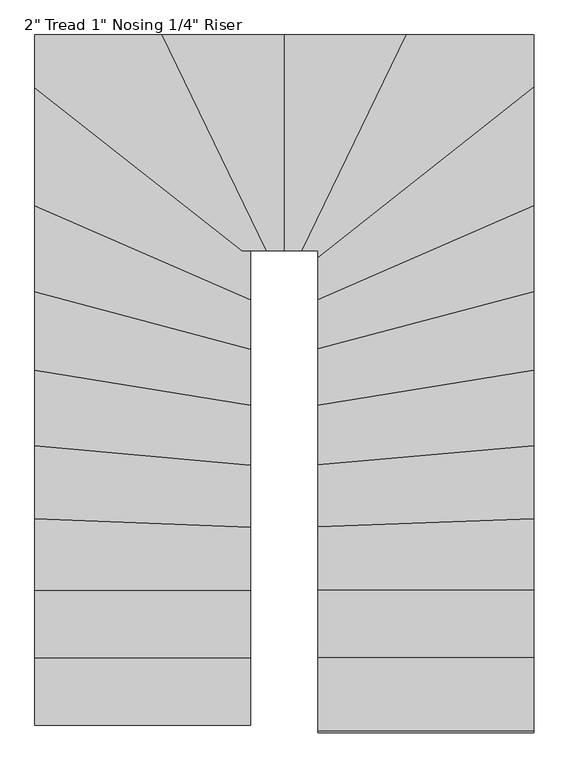
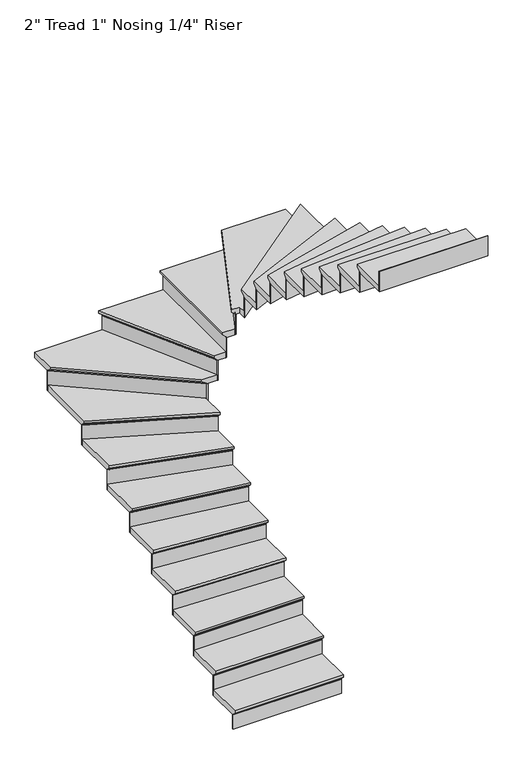
"""IFC4 building model written with IfcOpenShell, lengths in millimetres: stair flight geometry."""

from ifc_helpers import new_model, si_unit, origin, place, context, project, spatial, faceted_brep, source, transform, mapped, element, save


def stair_flight_652fc51c(model_context):
    return source(origin(), model_context, "Body", "Brep", [
        faceted_brep([(-5047.1987704, -4554.2130548, 22100.7214286), (-5047.1987704, -4554.2130548, 22119.7714286), (-5940.8822214, -4554.2130548, 22119.7714286), (-5940.8822214, -4554.2130548, 22100.7214286), (-5047.1987704, -4528.8130548, 22075.3214286), (-5940.8822214, -4528.8130548, 22075.3214286), (-5047.1987704, -4249.4130548, 22119.7714286), (-5940.8822214, -4249.4130548, 22119.7714286), (-5940.8822214, -4528.8130548, 22068.9714286), (-5940.8822214, -4249.4130548, 22068.9714286), (-5047.1987704, -4249.4130548, 22068.9714286), (-5047.1987704, -4528.8130548, 22068.9714286)], [[[0, 1, 2, 3]], [[4, 0, 3, 5]], [[2, 1, 6, 7]], [[8, 9, 10, 11]], [[2, 7, 9, 8, 5, 3]], [[8, 11, 4, 5]], [[6, 1, 0, 4, 11, 10]], [[7, 6, 10, 9]]]),
        faceted_brep([(-5047.1987704, -4528.8130548, 22068.9714286), (-5047.1987704, -4528.8130548, 21945.6), (-5047.1987704, -4522.4630548, 21945.6), (-5047.1987704, -4522.4630548, 22068.9714286), (-5940.8822214, -4528.8130548, 22068.9714286), (-5940.8822214, -4522.4630548, 22068.9714286), (-5940.8822214, -4522.4630548, 21945.6), (-5940.8822214, -4528.8130548, 21945.6)], [[[0, 1, 2, 3]], [[4, 5, 6, 7]], [[1, 0, 4, 7]], [[2, 1, 7, 6]], [[3, 2, 6, 5]], [[0, 3, 5, 4]]]),
        faceted_brep([(-5047.1987704, -4249.4130548, 22243.1428571), (-5047.1987704, -4249.4130548, 22068.9714286), (-5047.1987704, -4243.0630548, 22068.9714286), (-5047.1987704, -4243.0630548, 22243.1428571), (-5940.8822214, -4249.4130548, 22243.1428571), (-5940.8822214, -4243.0630548, 22243.1428571), (-5940.8822214, -4243.0630548, 22068.9714286), (-5940.8822214, -4249.4130548, 22068.9714286)], [[[0, 1, 2, 3]], [[4, 5, 6, 7]], [[1, 0, 4, 7]], [[2, 1, 7, 6]], [[3, 2, 6, 5]], [[0, 3, 5, 4]]]),
        faceted_brep([(-5940.8822214, -4274.8130548, 22293.9428571), (-5047.1987704, -4274.8130548, 22293.9428571), (-5047.1987704, -3970.0130548, 22293.9428571), (-5940.8822214, -3970.0130548, 22293.9428571), (-5940.8822214, -4249.4130548, 22243.1428571), (-5940.8822214, -3970.0130548, 22243.1428571), (-5047.1987704, -3970.0130548, 22243.1428571), (-5047.1987704, -4249.4130548, 22243.1428571), (-5940.8822214, -4249.4130548, 22249.4928571), (-5940.8822214, -4274.8130548, 22274.8928571), (-5047.1987704, -4249.4130548, 22249.4928571), (-5047.1987704, -4274.8130548, 22274.8928571)], [[[0, 1, 2, 3]], [[4, 5, 6, 7]], [[0, 3, 5, 4, 8, 9]], [[4, 7, 10, 8]], [[2, 1, 11, 10, 7, 6]], [[3, 2, 6, 5]], [[11, 1, 0, 9]], [[10, 11, 9, 8]]]),
        faceted_brep([(-5047.1987704, -3970.0130548, 22417.3142857), (-5047.1987704, -3970.0130548, 22243.1428571), (-5047.1987704, -3963.6630548, 22243.1428571), (-5047.1987704, -3963.6630548, 22417.3142857), (-5940.8822214, -3970.0130548, 22417.3142857), (-5940.8822214, -3963.6630548, 22417.3142857), (-5940.8822214, -3963.6630548, 22243.1428571), (-5940.8822214, -3970.0130548, 22243.1428571)], [[[0, 1, 2, 3]], [[4, 5, 6, 7]], [[1, 0, 4, 7]], [[2, 1, 7, 6]], [[3, 2, 6, 5]], [[0, 3, 5, 4]]]),
        faceted_brep([(-5940.8822214, -3995.4130548, 22468.1142857), (-5047.1987704, -3995.4130548, 22468.1142857), (-5047.1987704, -3707.9036879, 22468.1142857), (-5940.8822214, -3673.2843203, 22468.1142857), (-5940.8822214, -3970.0130548, 22417.3142857), (-5940.8822214, -3673.2843203, 22417.3142857), (-5047.1987704, -3707.9036879, 22417.3142857), (-5047.1987704, -3970.0130548, 22417.3142857), (-5940.8822214, -3970.0130548, 22423.6642857), (-5940.8822214, -3995.4130548, 22449.0642857), (-5047.1987704, -3970.0130548, 22423.6642857), (-5047.1987704, -3995.4130548, 22449.0642857)], [[[0, 1, 2, 3]], [[4, 5, 6, 7]], [[0, 3, 5, 4, 8, 9]], [[4, 7, 10, 8]], [[2, 1, 11, 10, 7, 6]], [[3, 2, 6, 5]], [[11, 1, 0, 9]], [[10, 11, 9, 8]]]),
        faceted_brep([(-5047.1987704, -3707.9036879, 22591.4857143), (-5047.1987704, -3707.9036879, 22417.3142857), (-5047.1987704, -3701.5489252, 22417.3142857), (-5047.1987704, -3701.5489252, 22591.4857143), (-5940.8822214, -3673.2843203, 22591.4857143), (-5940.8822214, -3666.9295576, 22591.4857143), (-5940.8822214, -3666.9295576, 22417.3142857), (-5940.8822214, -3673.2843203, 22417.3142857)], [[[0, 1, 2, 3]], [[4, 5, 6, 7]], [[1, 0, 4, 7]], [[2, 1, 7, 6]], [[3, 2, 6, 5]], [[0, 3, 5, 4]]]),
        faceted_brep([(-5940.8822214, -3698.703371, 22642.2857143), (-5047.1987704, -3733.3227386, 22642.2857143), (-5047.1987704, -3451.3234819, 22642.2857143), (-5940.8822214, -3370.89733, 22642.2857143), (-5940.8822214, -3673.2843203, 22591.4857143), (-5940.8822214, -3370.89733, 22591.4857143), (-5047.1987704, -3451.3234819, 22591.4857143), (-5047.1987704, -3707.9036879, 22591.4857143), (-5940.8822214, -3673.2843203, 22597.8357143), (-5940.8822214, -3698.703371, 22623.2357143), (-5047.1987704, -3707.9036879, 22597.8357143), (-5047.1987704, -3733.3227386, 22623.2357143)], [[[0, 1, 2, 3]], [[4, 5, 6, 7]], [[0, 3, 5, 4, 8, 9]], [[4, 7, 10, 8]], [[2, 1, 11, 10, 7, 6]], [[3, 2, 6, 5]], [[11, 1, 0, 9]], [[10, 11, 9, 8]]]),
        faceted_brep([(-5047.1987704, -3451.3234819, 22765.6571429), (-5047.1987704, -3451.3234819, 22591.4857143), (-5047.1987704, -3444.9478197, 22591.4857143), (-5047.1987704, -3444.9478197, 22765.6571429), (-5940.8822214, -3370.89733, 22765.6571429), (-5940.8822214, -3364.5216678, 22765.6571429), (-5940.8822214, -3364.5216678, 22591.4857143), (-5940.8822214, -3370.89733, 22591.4857143)], [[[0, 1, 2, 3]], [[4, 5, 6, 7]], [[1, 0, 4, 7]], [[2, 1, 7, 6]], [[3, 2, 6, 5]], [[0, 3, 5, 4]]]),
        faceted_brep([(-5940.8822214, -3396.3999789, 22816.4571429), (-5047.1987704, -3476.8261308, 22816.4571429), (-5047.1987704, -3203.4301079, 22816.4571429), (-5940.8822214, -3059.5417727, 22816.4571429), (-5940.8822214, -3370.89733, 22765.6571429), (-5940.8822214, -3059.5417727, 22765.6571429), (-5047.1987704, -3203.4301079, 22765.6571429), (-5047.1987704, -3451.3234819, 22765.6571429), (-5940.8822214, -3370.89733, 22772.0071429), (-5940.8822214, -3396.3999789, 22797.4071429), (-5047.1987704, -3451.3234819, 22772.0071429), (-5047.1987704, -3476.8261308, 22797.4071429)], [[[0, 1, 2, 3]], [[4, 5, 6, 7]], [[0, 3, 5, 4, 8, 9]], [[4, 7, 10, 8]], [[2, 1, 11, 10, 7, 6]], [[3, 2, 6, 5]], [[11, 1, 0, 9]], [[10, 11, 9, 8]]]),
        faceted_brep([(-5047.1987704, -3203.4301079, 22939.8285714), (-5047.1987704, -3203.4301079, 22765.6571429), (-5047.1987704, -3196.9983292, 22765.6571429), (-5047.1987704, -3196.9983292, 22939.8285714), (-5940.8822214, -3059.5417727, 22939.8285714), (-5940.8822214, -3053.109994, 22939.8285714), (-5940.8822214, -3053.109994, 22765.6571429), (-5940.8822214, -3059.5417727, 22765.6571429)], [[[0, 1, 2, 3]], [[4, 5, 6, 7]], [[1, 0, 4, 7]], [[2, 1, 7, 6]], [[3, 2, 6, 5]], [[0, 3, 5, 4]]]),
        faceted_brep([(-5940.8822214, -3085.2688872, 22990.6285714), (-5047.1987704, -3229.1572224, 22990.6285714), (-5047.1987704, -2970.3553609, 22990.6285714), (-5940.8822214, -2732.7052783, 22990.6285714), (-5940.8822214, -3059.5417727, 22939.8285714), (-5940.8822214, -2732.7052783, 22939.8285714), (-5047.1987704, -2970.3553609, 22939.8285714), (-5047.1987704, -3203.4301079, 22939.8285714), (-5940.8822214, -3059.5417727, 22946.1785714), (-5940.8822214, -3085.2688872, 22971.5785714), (-5047.1987704, -3203.4301079, 22946.1785714), (-5047.1987704, -3229.1572224, 22971.5785714)], [[[0, 1, 2, 3]], [[4, 5, 6, 7]], [[0, 3, 5, 4, 8, 9]], [[4, 7, 10, 8]], [[2, 1, 11, 10, 7, 6]], [[3, 2, 6, 5]], [[11, 1, 0, 9]], [[10, 11, 9, 8]]]),
        faceted_brep([(-5047.1987704, -2970.3553609, 23114.0), (-5047.1987704, -2970.3553609, 22939.8285714), (-5047.1987704, -2963.7846771, 22939.8285714), (-5047.1987704, -2963.7846771, 23114.0), (-5940.8822214, -2732.7052783, 23114.0), (-5940.8822214, -2726.1345945, 23114.0), (-5940.8822214, -2726.1345945, 22939.8285714), (-5940.8822214, -2732.7052783, 22939.8285714)], [[[0, 1, 2, 3]], [[4, 5, 6, 7]], [[1, 0, 4, 7]], [[2, 1, 7, 6]], [[3, 2, 6, 5]], [[0, 3, 5, 4]]]),
        faceted_brep([(-5940.8822214, -2758.9880136, 23164.8), (-5047.1987704, -2996.6380961, 23164.8), (-5047.1987704, -2765.8050203, 23164.8), (-5940.8822214, -2375.5896532, 23164.8), (-5940.8822214, -2732.7052783, 23114.0), (-5940.8822214, -2375.5896532, 23114.0), (-5047.1987704, -2765.8050203, 23114.0), (-5047.1987704, -2970.3553609, 23114.0), (-5940.8822214, -2732.7052783, 23120.35), (-5940.8822214, -2758.9880136, 23145.75), (-5047.1987704, -2970.3553609, 23120.35), (-5047.1987704, -2996.6380961, 23145.75)], [[[0, 1, 2, 3]], [[4, 5, 6, 7]], [[0, 3, 5, 4, 8, 9]], [[4, 7, 10, 8]], [[2, 1, 11, 10, 7, 6]], [[3, 2, 6, 5]], [[11, 1, 0, 9]], [[10, 11, 9, 8]]]),
        faceted_brep([(-5047.1987704, -2765.8050203, 23288.1714286), (-5047.1987704, -2765.8050203, 23114.0), (-5047.1987704, -2758.8760908, 23114.0), (-5047.1987704, -2758.8760908, 23288.1714286), (-5940.8822214, -2375.5896532, 23288.1714286), (-5940.8822214, -2368.6607237, 23288.1714286), (-5940.8822214, -2368.6607237, 23114.0), (-5940.8822214, -2375.5896532, 23114.0)], [[[0, 1, 2, 3]], [[4, 5, 6, 7]], [[1, 0, 4, 7]], [[2, 1, 7, 6]], [[3, 2, 6, 5]], [[0, 3, 5, 4]]]),
        faceted_brep([(-5940.8822214, -2403.3053713, 23338.9714286), (-5047.1987704, -2793.5207384, 23338.9714286), (-5047.1987704, -2590.8424524, 23338.9714286), (-5040.8038639, -2590.8424524, 23338.9714286), (-5940.8822214, -1882.1944717, 23338.9714286), (-5940.8822214, -2375.5896532, 23288.1714286), (-5940.8822214, -1882.1944717, 23288.1714286), (-5040.8038639, -2590.8424524, 23288.1714286), (-5047.1987704, -2590.8424524, 23288.1714286), (-5047.1987704, -2765.8050203, 23288.1714286), (-5940.8822214, -2375.5896532, 23294.5214286), (-5940.8822214, -2403.3053713, 23319.9214286), (-5047.1987704, -2765.8050203, 23294.5214286), (-5047.1987704, -2793.5207384, 23319.9214286)], [[[0, 1, 2, 3, 4]], [[5, 6, 7, 8, 9]], [[0, 4, 6, 5, 10, 11]], [[5, 9, 12, 10]], [[2, 1, 13, 12, 9, 8]], [[4, 3, 7, 6]], [[13, 1, 0, 11]], [[12, 13, 11, 10]], [[3, 2, 8, 7]]]),
        faceted_brep([(-5040.8038639, -2590.8424524, 23462.3428571), (-5040.8038639, -2590.8424524, 23288.1714286), (-5030.5387554, -2590.8424524, 23288.1714286), (-5030.5387554, -2590.8424524, 23462.3428571), (-5940.8822214, -1882.1944717, 23462.3428571), (-5940.8822214, -1874.1125661, 23462.3428571), (-5940.8822214, -1874.1125661, 23288.1714286), (-5940.8822214, -1882.1944717, 23288.1714286)], [[[0, 1, 2, 3]], [[4, 5, 6, 7]], [[1, 0, 4, 7]], [[2, 1, 7, 6]], [[3, 2, 6, 5]], [[0, 3, 5, 4]]]),
        faceted_brep([(-5384.6489457, -1697.1590014, 23513.1428571), (-5940.8822214, -1697.1590014, 23513.1428571), (-5940.8822214, -1914.5220945, 23513.1428571), (-5081.8642978, -2590.8424524, 23513.1428571), (-4952.3566185, -2590.8424524, 23513.1428571), (-5940.8822214, -1697.1590014, 23462.3428571), (-5384.6489457, -1697.1590014, 23462.3428571), (-4952.3566185, -2590.8424524, 23462.3428571), (-5040.8038639, -2590.8424524, 23462.3428571), (-5940.8822214, -1882.1944717, 23462.3428571), (-5940.8822214, -1882.1944717, 23468.6928571), (-5940.8822214, -1914.5220945, 23494.0928571), (-5040.8038639, -2590.8424524, 23468.6928571), (-5081.8642978, -2590.8424524, 23494.0928571)], [[[0, 1, 2, 3, 4]], [[5, 6, 7, 8, 9]], [[1, 0, 6, 5]], [[2, 1, 5, 9, 10, 11]], [[9, 8, 12, 10]], [[4, 3, 13, 12, 8, 7]], [[0, 4, 7, 6]], [[13, 3, 2, 11]], [[12, 13, 11, 10]]]),
        faceted_brep([(-4952.3566185, -2590.8424524, 23636.5142857), (-4952.3566185, -2590.8424524, 23462.3428571), (-4945.3027294, -2590.8424524, 23462.3428571), (-4945.3027294, -2590.8424524, 23636.5142857), (-5384.6489457, -1697.1590014, 23636.5142857), (-5377.5950566, -1697.1590014, 23636.5142857), (-5377.5950566, -1697.1590014, 23462.3428571), (-5384.6489457, -1697.1590014, 23462.3428571)], [[[0, 1, 2, 3]], [[4, 5, 6, 7]], [[1, 0, 4, 7]], [[2, 1, 7, 6]], [[3, 2, 6, 5]], [[0, 3, 5, 4]]]),
        faceted_brep([(-5412.8645022, -1697.1590014, 23687.3142857), (-4980.5721749, -2590.8424524, 23687.3142857), (-4882.0987704, -2590.8424524, 23687.3142857), (-4882.0987706, -1697.1590014, 23687.3142857), (-5384.6489457, -1697.1590014, 23636.5142857), (-4882.0987706, -1697.1590014, 23636.5142857), (-4882.0987704, -2590.8424524, 23636.5142857), (-4952.3566185, -2590.8424524, 23636.5142857), (-5384.6489457, -1697.1590014, 23642.8642857), (-5412.8645022, -1697.1590014, 23668.2642857), (-4952.3566185, -2590.8424524, 23642.8642857), (-4980.5721749, -2590.8424524, 23668.2642857)], [[[0, 1, 2, 3]], [[4, 5, 6, 7]], [[0, 3, 5, 4, 8, 9]], [[4, 7, 10, 8]], [[3, 2, 6, 5]], [[11, 1, 0, 9]], [[10, 11, 9, 8]], [[2, 1, 11, 10, 7, 6]]]),
        faceted_brep([(-4882.0987704, -2590.8424524, 23810.6857143), (-4882.0987704, -2590.8424524, 23636.5142857), (-4875.7487704, -2590.8424524, 23636.5142857), (-4875.7487704, -2590.8424524, 23810.6857143), (-4882.0987706, -1697.1590014, 23810.6857143), (-4875.7487706, -1697.1590014, 23810.6857143), (-4875.7487706, -1697.1590014, 23636.5142857), (-4882.0987706, -1697.1590014, 23636.5142857)], [[[0, 1, 2, 3]], [[4, 5, 6, 7]], [[1, 0, 4, 7]], [[2, 1, 7, 6]], [[3, 2, 6, 5]], [[0, 3, 5, 4]]]),
        faceted_brep([(-4907.4987706, -1697.1590014, 23861.4857143), (-4907.4987704, -2590.8424524, 23861.4857143), (-4806.2098095, -2590.8424524, 23861.4857143), (-4373.9174828, -1697.1590014, 23861.4857143), (-4882.0987706, -1697.1590014, 23810.6857143), (-4373.9174828, -1697.1590014, 23810.6857143), (-4806.2098095, -2590.8424524, 23810.6857143), (-4882.0987704, -2590.8424524, 23810.6857143), (-4882.0987706, -1697.1590014, 23817.0357143), (-4907.4987706, -1697.1590014, 23842.4357143), (-4882.0987704, -2590.8424524, 23817.0357143), (-4907.4987704, -2590.8424524, 23842.4357143)], [[[0, 1, 2, 3]], [[4, 5, 6, 7]], [[0, 3, 5, 4, 8, 9]], [[4, 7, 10, 8]], [[2, 1, 11, 10, 7, 6]], [[3, 2, 6, 5]], [[11, 1, 0, 9]], [[10, 11, 9, 8]]]),
        faceted_brep([(-4806.2098095, -2590.8424524, 23984.8571429), (-4806.2098095, -2590.8424524, 23810.6857143), (-4799.1559204, -2590.8424524, 23810.6857143), (-4799.1559204, -2590.8424524, 23984.8571429), (-4373.9174828, -1697.1590014, 23984.8571429), (-4366.8635937, -1697.1590014, 23984.8571429), (-4366.8635937, -1697.1590014, 23810.6857143), (-4373.9174828, -1697.1590014, 23810.6857143)], [[[0, 1, 2, 3]], [[4, 5, 6, 7]], [[1, 0, 4, 7]], [[2, 1, 7, 6]], [[3, 2, 6, 5]], [[0, 3, 5, 4]]]),
        faceted_brep([(-3874.1153195, -1946.8497166, 24035.6571429), (-3874.1153195, -1697.1590014, 24035.6571429), (-4402.1330392, -1697.1590014, 24035.6571429), (-4834.4253659, -2590.8424524, 24035.6571429), (-4767.7987704, -2590.8424524, 24035.6571429), (-4767.7987704, -2650.4628721, 24035.6571429), (-3874.1153195, -1697.1590014, 23984.8571429), (-3874.1153195, -1946.8497166, 23984.8571429), (-4767.7987704, -2650.4628721, 23984.8571429), (-4767.7987704, -2590.8424524, 23984.8571429), (-4806.2098095, -2590.8424524, 23984.8571429), (-4373.9174828, -1697.1590014, 23984.8571429), (-4806.2098095, -2590.8424524, 23991.2071429), (-4373.9174828, -1697.1590014, 23991.2071429), (-4834.4253659, -2590.8424524, 24016.6071429), (-4402.1330392, -1697.1590014, 24016.6071429)], [[[0, 1, 2, 3, 4, 5]], [[6, 7, 8, 9, 10, 11]], [[1, 0, 7, 6]], [[11, 10, 12, 13]], [[4, 3, 14, 12, 10, 9]], [[5, 4, 9, 8]], [[0, 5, 8, 7]], [[14, 3, 2, 15]], [[12, 14, 15, 13]], [[2, 1, 6, 11, 13, 15]]]),
        faceted_brep([(-4767.7987704, -2650.4628721, 24159.0285714), (-4767.7987704, -2650.4628721, 23984.8571429), (-4767.7987704, -2658.5447778, 23984.8571429), (-4767.7987704, -2658.5447778, 24159.0285714), (-3874.1153195, -1946.8497166, 24159.0285714), (-3874.1153195, -1954.9316222, 24159.0285714), (-3874.1153195, -1954.9316222, 23984.8571429), (-3874.1153195, -1946.8497166, 23984.8571429)], [[[0, 1, 2, 3]], [[4, 5, 6, 7]], [[1, 0, 4, 7]], [[2, 1, 7, 6]], [[3, 2, 6, 5]], [[0, 3, 5, 4]]]),
        faceted_brep([(-3874.1153195, -1914.5220938, 24209.8285714), (-4767.7987704, -2618.1352494, 24209.8285714), (-4767.7987704, -2821.2364563, 24209.8285714), (-3874.1153195, -2431.0210889, 24209.8285714), (-3874.1153195, -1946.8497166, 24159.0285714), (-3874.1153195, -2431.0210889, 24159.0285714), (-4767.7987704, -2821.2364563, 24159.0285714), (-4767.7987704, -2650.4628721, 24159.0285714), (-3874.1153195, -1946.8497166, 24165.3785714), (-3874.1153195, -1914.5220938, 24190.7785714), (-4767.7987704, -2650.4628721, 24165.3785714), (-4767.7987704, -2618.1352494, 24190.7785714)], [[[0, 1, 2, 3]], [[4, 5, 6, 7]], [[0, 3, 5, 4, 8, 9]], [[4, 7, 10, 8]], [[2, 1, 11, 10, 7, 6]], [[3, 2, 6, 5]], [[11, 1, 0, 9]], [[10, 11, 9, 8]]]),
        faceted_brep([(-4767.7987704, -2821.2364563, 24333.2), (-4767.7987704, -2821.2364563, 24159.0285714), (-4767.7987704, -2828.1653858, 24159.0285714), (-4767.7987704, -2828.1653858, 24333.2), (-3874.1153195, -2431.0210889, 24333.2), (-3874.1153195, -2437.9500185, 24333.2), (-3874.1153195, -2437.9500185, 24159.0285714), (-3874.1153195, -2431.0210889, 24159.0285714)], [[[0, 1, 2, 3]], [[4, 5, 6, 7]], [[1, 0, 4, 7]], [[2, 1, 7, 6]], [[3, 2, 6, 5]], [[0, 3, 5, 4]]]),
        faceted_brep([(-3874.1153195, -2403.3053709, 24384.0), (-4767.7987704, -2793.5207382, 24384.0), (-4767.7987704, -3022.9208311, 24384.0), (-3874.1153195, -2785.2707484, 24384.0), (-3874.1153195, -2431.0210889, 24333.2), (-3874.1153195, -2785.2707484, 24333.2), (-4767.7987704, -3022.9208311, 24333.2), (-4767.7987704, -2821.2364563, 24333.2), (-3874.1153195, -2431.0210889, 24339.55), (-3874.1153195, -2403.3053709, 24364.95), (-4767.7987704, -2821.2364563, 24339.55), (-4767.7987704, -2793.5207382, 24364.95)], [[[0, 1, 2, 3]], [[4, 5, 6, 7]], [[0, 3, 5, 4, 8, 9]], [[4, 7, 10, 8]], [[2, 1, 11, 10, 7, 6]], [[3, 2, 6, 5]], [[11, 1, 0, 9]], [[10, 11, 9, 8]]]),
        faceted_brep([(-4767.7987704, -3022.9208311, 24507.3714286), (-4767.7987704, -3022.9208311, 24333.2), (-4767.7987704, -3029.4915149, 24333.2), (-4767.7987704, -3029.4915149, 24507.3714286), (-3874.1153195, -2785.2707484, 24507.3714286), (-3874.1153195, -2791.8414322, 24507.3714286), (-3874.1153195, -2791.8414322, 24333.2), (-3874.1153195, -2785.2707484, 24333.2)], [[[0, 1, 2, 3]], [[4, 5, 6, 7]], [[1, 0, 4, 7]], [[2, 1, 7, 6]], [[3, 2, 6, 5]], [[0, 3, 5, 4]]]),
        faceted_brep([(-3874.1153195, -2758.9880132, 24558.1714286), (-4767.7987704, -2996.6380959, 24558.1714286), (-4767.7987704, -3254.8843368, 24558.1714286), (-3874.1153195, -3110.9960015, 24558.1714286), (-3874.1153195, -2785.2707484, 24507.3714286), (-3874.1153195, -3110.9960015, 24507.3714286), (-4767.7987704, -3254.8843368, 24507.3714286), (-4767.7987704, -3022.9208311, 24507.3714286), (-3874.1153195, -2785.2707484, 24513.7214286), (-3874.1153195, -2758.9880132, 24539.1214286), (-4767.7987704, -3022.9208311, 24513.7214286), (-4767.7987704, -2996.6380959, 24539.1214286)], [[[0, 1, 2, 3]], [[4, 5, 6, 7]], [[0, 3, 5, 4, 8, 9]], [[4, 7, 10, 8]], [[2, 1, 11, 10, 7, 6]], [[3, 2, 6, 5]], [[11, 1, 0, 9]], [[10, 11, 9, 8]]]),
        faceted_brep([(-4767.7987704, -3254.8843368, 24681.5428571), (-4767.7987704, -3254.8843368, 24507.3714286), (-4767.7987704, -3261.3161154, 24507.3714286), (-4767.7987704, -3261.3161154, 24681.5428571), (-3874.1153195, -3110.9960015, 24681.5428571), (-3874.1153195, -3117.4277801, 24681.5428571), (-3874.1153195, -3117.4277801, 24507.3714286), (-3874.1153195, -3110.9960015, 24507.3714286)], [[[0, 1, 2, 3]], [[4, 5, 6, 7]], [[1, 0, 4, 7]], [[2, 1, 7, 6]], [[3, 2, 6, 5]], [[0, 3, 5, 4]]]),
        faceted_brep([(-3874.1153195, -3085.2688869, 24732.3428571), (-4767.7987704, -3229.1572222, 24732.3428571), (-4767.7987704, -3502.3287795, 24732.3428571), (-3874.1153195, -3421.9026274, 24732.3428571), (-3874.1153195, -3110.9960015, 24681.5428571), (-3874.1153195, -3421.9026274, 24681.5428571), (-4767.7987704, -3502.3287795, 24681.5428571), (-4767.7987704, -3254.8843368, 24681.5428571), (-3874.1153195, -3110.9960015, 24687.8928571), (-3874.1153195, -3085.2688869, 24713.2928571), (-4767.7987704, -3254.8843368, 24687.8928571), (-4767.7987704, -3229.1572222, 24713.2928571)], [[[0, 1, 2, 3]], [[4, 5, 6, 7]], [[0, 3, 5, 4, 8, 9]], [[4, 7, 10, 8]], [[2, 1, 11, 10, 7, 6]], [[3, 2, 6, 5]], [[11, 1, 0, 9]], [[10, 11, 9, 8]]]),
        faceted_brep([(-4767.7987704, -3502.3287795, 24855.7142857), (-4767.7987704, -3502.3287795, 24681.5428571), (-4767.7987704, -3508.7044417, 24681.5428571), (-4767.7987704, -3508.7044417, 24855.7142857), (-3874.1153195, -3421.9026274, 24855.7142857), (-3874.1153195, -3428.2782897, 24855.7142857), (-3874.1153195, -3428.2782897, 24681.5428571), (-3874.1153195, -3421.9026274, 24681.5428571)], [[[0, 1, 2, 3]], [[4, 5, 6, 7]], [[1, 0, 4, 7]], [[2, 1, 7, 6]], [[3, 2, 6, 5]], [[0, 3, 5, 4]]]),
        faceted_brep([(-3874.1153195, -3396.3999786, 24906.5142857), (-4767.7987704, -3476.8261306, 24906.5142857), (-4767.7987704, -3758.7417891, 24906.5142857), (-3874.1153195, -3724.1224215, 24906.5142857), (-3874.1153195, -3421.9026274, 24855.7142857), (-3874.1153195, -3724.1224215, 24855.7142857), (-4767.7987704, -3758.7417891, 24855.7142857), (-4767.7987704, -3502.3287795, 24855.7142857), (-3874.1153195, -3421.9026274, 24862.0642857), (-3874.1153195, -3396.3999786, 24887.4642857), (-4767.7987704, -3502.3287795, 24862.0642857), (-4767.7987704, -3476.8261306, 24887.4642857)], [[[0, 1, 2, 3]], [[4, 5, 6, 7]], [[0, 3, 5, 4, 8, 9]], [[4, 7, 10, 8]], [[2, 1, 11, 10, 7, 6]], [[3, 2, 6, 5]], [[11, 1, 0, 9]], [[10, 11, 9, 8]]]),
        faceted_brep([(-4767.7987704, -3758.7417891, 25029.8857143), (-4767.7987704, -3758.7417891, 24855.7142857), (-4767.7987704, -3765.0965518, 24855.7142857), (-4767.7987704, -3765.0965518, 25029.8857143), (-3874.1153195, -3724.1224215, 25029.8857143), (-3874.1153195, -3730.4771842, 25029.8857143), (-3874.1153195, -3730.4771842, 24855.7142857), (-3874.1153195, -3724.1224215, 24855.7142857)], [[[0, 1, 2, 3]], [[4, 5, 6, 7]], [[1, 0, 4, 7]], [[2, 1, 7, 6]], [[3, 2, 6, 5]], [[0, 3, 5, 4]]]),
        faceted_brep([(-3874.1153195, -3698.7033708, 25080.6857143), (-4767.7987704, -3733.3227384, 25080.6857143), (-4767.7987704, -4020.8130546, 25080.6857143), (-3874.1153195, -4020.8130546, 25080.6857143), (-3874.1153195, -3724.1224215, 25029.8857143), (-3874.1153195, -4020.8130546, 25029.8857143), (-4767.7987704, -4020.8130546, 25029.8857143), (-4767.7987704, -3758.7417891, 25029.8857143), (-3874.1153195, -3724.1224215, 25036.2357143), (-3874.1153195, -3698.7033708, 25061.6357143), (-4767.7987704, -3758.7417891, 25036.2357143), (-4767.7987704, -3733.3227384, 25061.6357143)], [[[0, 1, 2, 3]], [[4, 5, 6, 7]], [[0, 3, 5, 4, 8, 9]], [[4, 7, 10, 8]], [[2, 1, 11, 10, 7, 6]], [[3, 2, 6, 5]], [[11, 1, 0, 9]], [[10, 11, 9, 8]]]),
        faceted_brep([(-4767.7987704, -4020.8130546, 25204.0571429), (-4767.7987704, -4020.8130546, 25029.8857143), (-4767.7987704, -4027.1630546, 25029.8857143), (-4767.7987704, -4027.1630546, 25204.0571429), (-3874.1153195, -4020.8130546, 25204.0571429), (-3874.1153195, -4027.1630546, 25204.0571429), (-3874.1153195, -4027.1630546, 25029.8857143), (-3874.1153195, -4020.8130546, 25029.8857143)], [[[0, 1, 2, 3]], [[4, 5, 6, 7]], [[1, 0, 4, 7]], [[2, 1, 7, 6]], [[3, 2, 6, 5]], [[0, 3, 5, 4]]]),
        faceted_brep([(-3874.1153195, -3995.4130546, 25254.8571429), (-4767.7987704, -3995.4130546, 25254.8571429), (-4767.7987704, -4300.2130546, 25254.8571429), (-3874.1153195, -4300.2130546, 25254.8571429), (-3874.1153195, -4020.8130546, 25204.0571429), (-3874.1153195, -4300.2130546, 25204.0571429), (-4767.7987704, -4300.2130546, 25204.0571429), (-4767.7987704, -4020.8130546, 25204.0571429), (-3874.1153195, -4020.8130546, 25210.4071429), (-3874.1153195, -3995.4130546, 25235.8071429), (-4767.7987704, -4020.8130546, 25210.4071429), (-4767.7987704, -3995.4130546, 25235.8071429)], [[[0, 1, 2, 3]], [[4, 5, 6, 7]], [[0, 3, 5, 4, 8, 9]], [[4, 7, 10, 8]], [[2, 1, 11, 10, 7, 6]], [[3, 2, 6, 5]], [[11, 1, 0, 9]], [[10, 11, 9, 8]]]),
        faceted_brep([(-4767.7987704, -4300.2130546, 25378.2285714), (-4767.7987704, -4300.2130546, 25204.0571429), (-4767.7987704, -4306.5630546, 25204.0571429), (-4767.7987704, -4306.5630546, 25378.2285714), (-3874.1153195, -4300.2130546, 25378.2285714), (-3874.1153195, -4306.5630546, 25378.2285714), (-3874.1153195, -4306.5630546, 25204.0571429), (-3874.1153195, -4300.2130546, 25204.0571429)], [[[0, 1, 2, 3]], [[4, 5, 6, 7]], [[1, 0, 4, 7]], [[2, 1, 7, 6]], [[3, 2, 6, 5]], [[0, 3, 5, 4]]]),
        faceted_brep([(-4767.7987704, -4579.6130546, 25552.4), (-4767.7987704, -4579.6130546, 25378.2285714), (-4767.7987704, -4585.9630546, 25378.2285714), (-4767.7987704, -4585.9630546, 25552.4), (-3874.1153195, -4579.6130546, 25552.4), (-3874.1153195, -4585.9630546, 25552.4), (-3874.1153195, -4585.9630546, 25378.2285714), (-3874.1153195, -4579.6130546, 25378.2285714)], [[[0, 1, 2, 3]], [[4, 5, 6, 7]], [[1, 0, 4, 7]], [[2, 1, 7, 6]], [[3, 2, 6, 5]], [[0, 3, 5, 4]]]),
        faceted_brep([(-3874.1153195, -4274.8130546, 25429.0285714), (-4767.7987704, -4274.8130546, 25429.0285714), (-4767.7987704, -4579.6130546, 25429.0285714), (-3874.1153195, -4579.6130546, 25429.0285714), (-3874.1153195, -4300.2130546, 25378.2285714), (-3874.1153195, -4579.6130546, 25378.2285714), (-4767.7987704, -4579.6130546, 25378.2285714), (-4767.7987704, -4300.2130546, 25378.2285714), (-3874.1153195, -4300.2130546, 25384.5785714), (-3874.1153195, -4274.8130546, 25409.9785714), (-4767.7987704, -4300.2130546, 25384.5785714), (-4767.7987704, -4274.8130546, 25409.9785714)], [[[0, 1, 2, 3]], [[4, 5, 6, 7]], [[0, 3, 5, 4, 8, 9]], [[4, 7, 10, 8]], [[2, 1, 11, 10, 7, 6]], [[3, 2, 6, 5]], [[11, 1, 0, 9]], [[10, 11, 9, 8]]]),
    ])


if __name__ == "__main__":
    model = new_model("IFC4")
    model_context = context("Model", 3, world=origin())
    ifc_project = project(units=[si_unit("LENGTHUNIT", "METRE", prefix="MILLI")], contexts=[model_context])
    site = spatial("IfcSite", under=ifc_project)
    building = spatial("IfcBuilding", under=site)
    placement = place(None, origin())
    stair_flight_shape = stair_flight_652fc51c(model_context)
    element("IfcStairFlight", 1, ObjectType="2\" Tread 1\" Nosing 1/4\" Riser", at=placement, inside=building, context=model_context, shape_type="MappedRepresentation", body=[
        mapped(stair_flight_shape, transform((0.0, 0.0, 0.0), x_axis=(1.0, 0.0, 0.0), y_axis=(0.0, 1.0, 0.0), z_axis=(0.0, 0.0, 1.0))),
    ])
    save(model, "model.ifc")

# Revit data of these elements
# Element 1 (IfcStairFlight, "2\" Tread 1\" Nosing 1/4\" Riser")
#   Materials on its faces: "Tile, Porcelain, 4in"
# Materials
#   "Tile, Porcelain, 4in": class "Generic", colour RGB 89 87 158, transparency 0, Description = "Porcelain tile, 4\", white", Cost = 0
